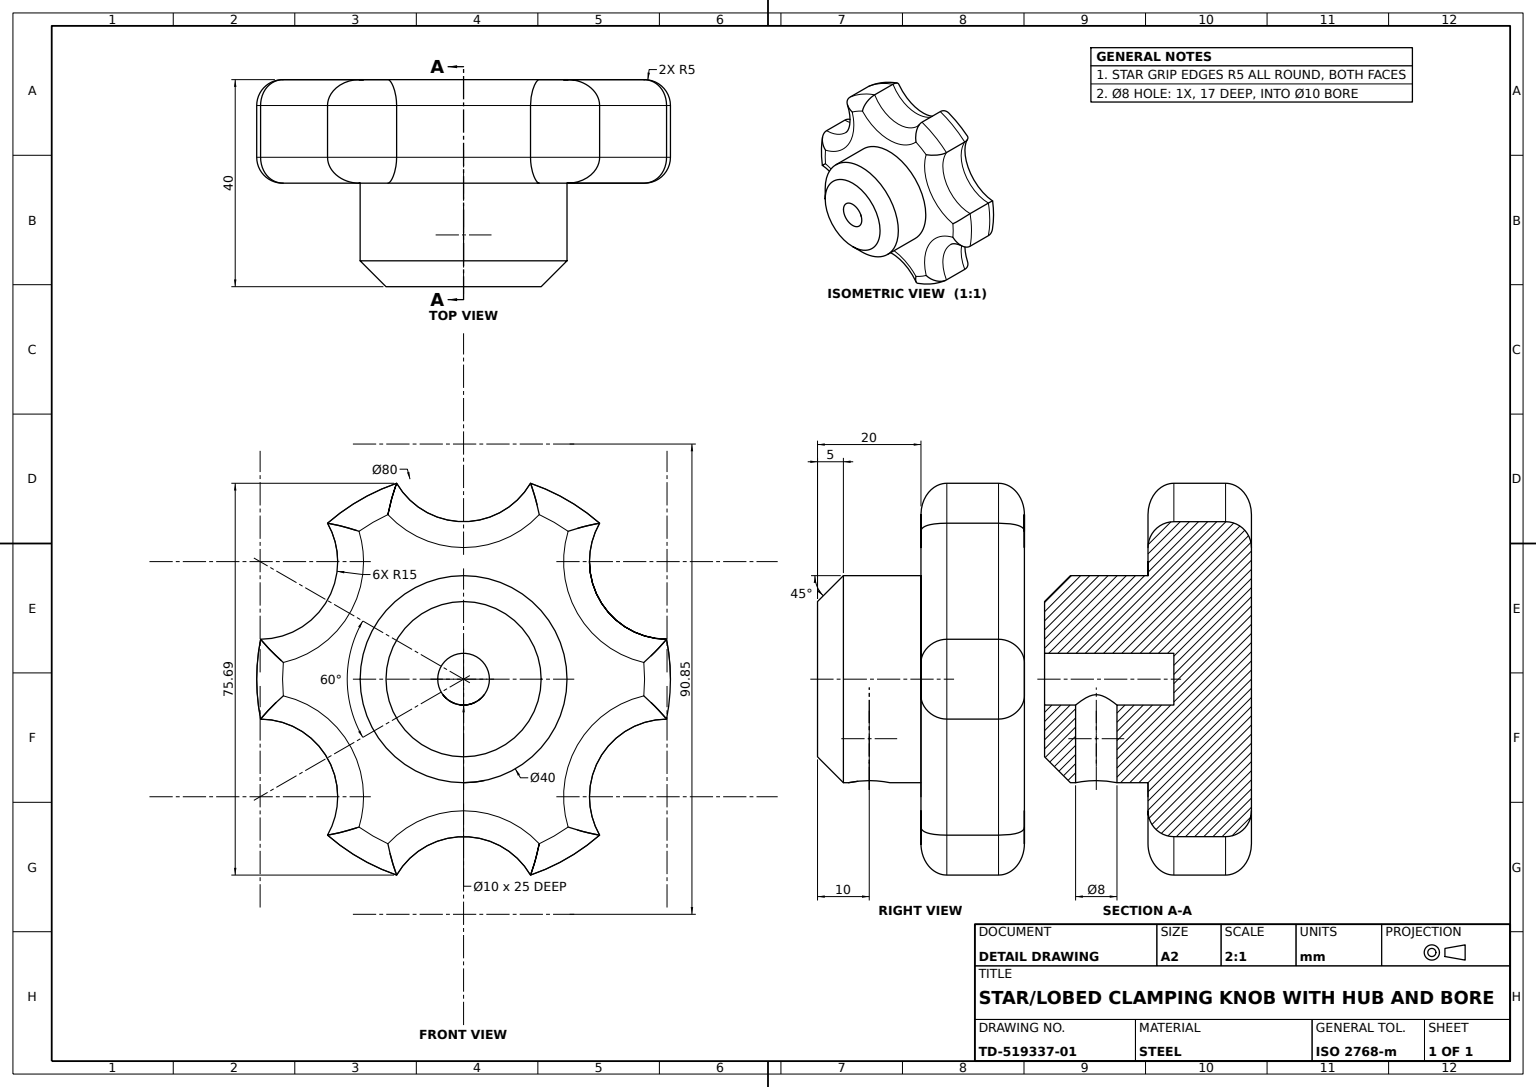
SolidWorks part; units mm, degrees
material "Plain Carbon Steel"
ref_plane "Front Plane" through (0, 0, 0) normal (0, 0, 1) x (1, 0, 0)
ref_plane "Top Plane" through (0, 0, 0) normal (0, 1, 0) x (1, 0, 0)
ref_plane "Right Plane" through (0, 0, 0) normal (1, 0, 0) x (0, 0, -1)
sketch "Star Grip Profile Sketch" plane through (0, 0, 0) normal (0, 0, 1) x (1, 0, 0)
  line L0 (-56.9243, 0) -> (88.9799, 0) construction
  line L1 (0, 61.6071) -> (0, -57.1303) construction
  arc A0 (-39.2493, 7.7129) -> (-39.2493, -7.7129) centre (0, 0) ccw
  arc A1 (12.9451, 37.8474) -> (-12.9451, 37.8474) centre (0, 45.4253) cw
  arc A2 (39.2493, 7.7129) -> (26.3043, 30.1345) centre (39.3395, 22.7127) cw
  arc A3 (26.3043, -30.1345) -> (39.2493, -7.7129) centre (39.3395, -22.7127) cw
  arc A4 (-12.9451, -37.8474) -> (12.9451, -37.8474) centre (0, -45.4253) cw
  arc A5 (-39.2493, -7.7129) -> (-26.3043, -30.1345) centre (-39.3395, -22.7127) cw
  arc A6 (-26.3043, 30.1345) -> (-39.2493, 7.7129) centre (-39.3395, 22.7127) cw
  arc A7 (-12.9451, 37.8474) -> (-26.3043, 30.1345) centre (0, 0) ccw
  arc A8 (26.3043, 30.1345) -> (12.9451, 37.8474) centre (0, 0) ccw
  arc A9 (39.2493, -7.7129) -> (39.2493, 7.7129) centre (0, 0) ccw
  arc A10 (12.9451, -37.8474) -> (26.3043, -30.1345) centre (0, 0) ccw
  arc A11 (-26.3043, -30.1345) -> (-12.9451, -37.8474) centre (0, 0) ccw
  point P28 (0, 0)
  dimension "D1" = 80
  dimension "D2" = 15
  dimension "D3" = 12.9451
  dimension "D4" = 6
extrude "Star Grip Body" add sketch "Star Grip Profile Sketch" along normal blind 20
sketch "Hub Sketch" plane through (0, 0, 20) normal (0, 0, 1) x (1, 0, 0)
  circle A0 centre (0, 0) radius 20
  circle A1 centre (0, 0) radius 17.5
  dimension "D1" = 40
  dimension "D2" = 35
extrude "Hub Boss Ø40" add sketch "Hub Sketch" along normal blind 20 contours A0 A1 | A1
sketch "Bore Sketch" plane through (0, 0, 40) normal (0, 0, 1) x (1, 0, 0)
  circle A0 centre (0, 0) radius 5
  dimension "D1" = 10
extrude "Axial Bore Ø10" cut sketch "Bore Sketch" against normal blind 25
sketch "Set Screw Hole Sketch" plane through (0, 0, 0) normal (0, 1, 0) x (1, 0, 0)
  circle A0 centre (0, -30) radius 4
  dimension "D1" = 8
  dimension "D2" = 30
extrude "Set Screw Hole Ø8" cut sketch "Set Screw Hole Sketch" against normal blind 24
chamfer "Hub Chamfer 5x45" distance 5 angle 45 1 edges at (20, 0, 40)
fillet "Grip Edge Fillet R5 A" radius 5 12 edges at (-20, 34.641, 20) (-26.3491, 15.2127, 20) (-40, 0, 20) (-26.3491, -15.2127, 20) (-20, -34.641, 20) (0, -30.4253, 20) (0, 30.4253, 20) (20, 34.641, 20) (26.3491, 15.2127, 20) (40, 0, 20) (26.3491, -15.2127, 20) (20, -34.641, 20)
fillet "Grip Edge Fillet R5 B" radius 5 12 edges at (0, 30.4253, 0) (-20, 34.641, 0) (-26.3491, 15.2127, 0) (-40, 0, 0) (-26.3491, -15.2127, 0) (-20, -34.641, 0) (0, -30.4253, 0) (20, -34.641, 0) (26.3491, -15.2127, 0) (40, 0, 0) (26.3491, 15.2127, 0) (20, 34.641, 0)
